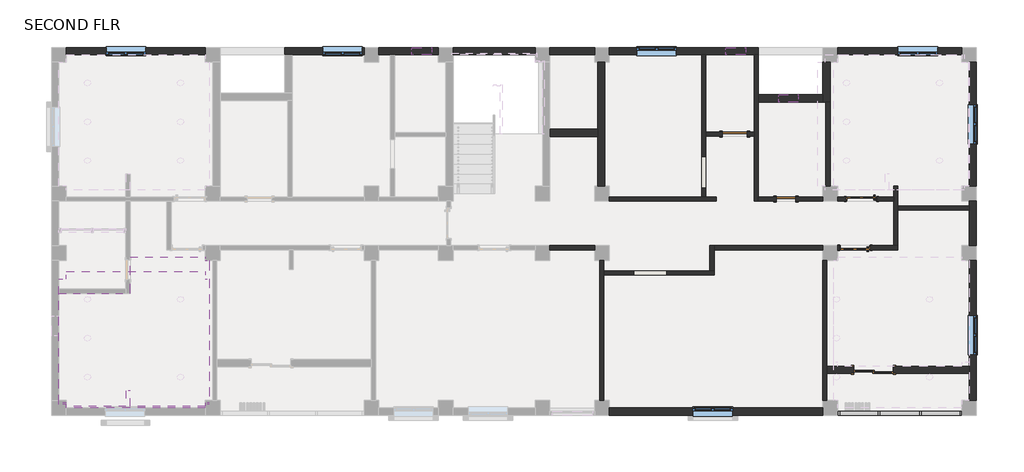
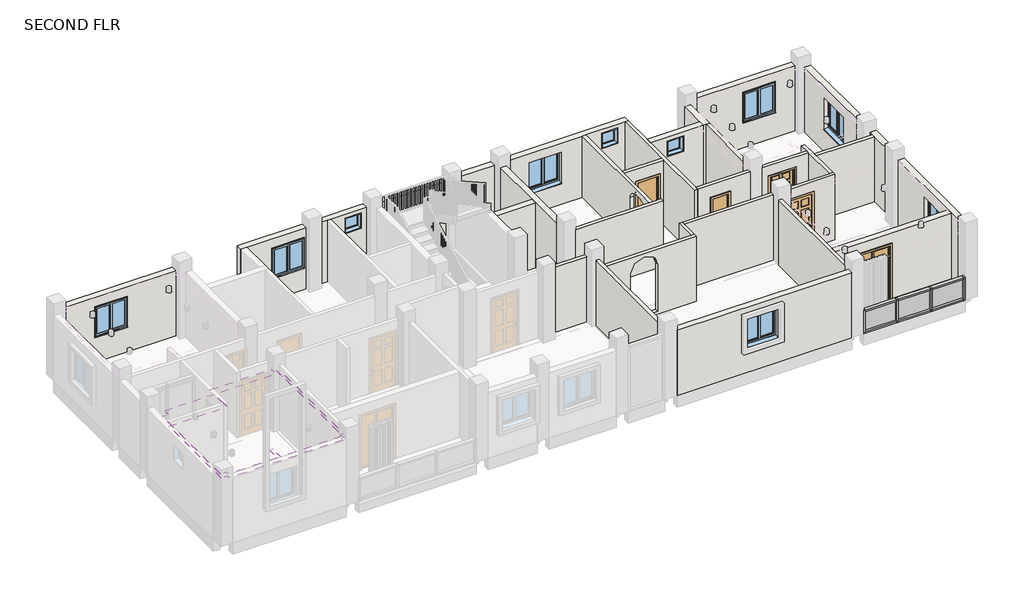
# One storey, part 2 of 5: 32 walls, 10 members, 10 windows, 5 doors, 3 plates, 2 coverings.
# Revit data of these elements (continued)
# Element 60 (IfcWindow, "w2.0001 : 4' X 4' WINDOW") (continued)
#   Materials on its faces: "Fenster - Kunststoff", "Fenster - Kunststoff weiss", "Glass", "Fenster - Holz"
# Element 61 (IfcWindow, "w2.0001 : 4' X 4' WINDOW")
#   Mark = "100"
#   Einbautiefe (von außen) = 0' - 5.51181"
#   Kippflügel = yes
#   Drehflügel im Grundriß darstellen = no
#   Drehflügel = yes
#   Rahmen = none
#   Glas = none
#   Flügel = none
#   Fensterbank innen = none
#   Fensterbank aussen = none
#   Phase Created = New Construction
#   Materials on its faces: "Fenster - Kunststoff", "Fenster - Kunststoff weiss", "Glass", "Fenster - Holz"
# Element 62 (IfcWindow, "w2.0001 : 4' X 4' WINDOW")
#   Mark = "106"
#   Einbautiefe (von außen) = 0' - 5.51181"
#   Kippflügel = yes
#   Drehflügel im Grundriß darstellen = no
#   Drehflügel = yes
#   Rahmen = none
#   Glas = none
#   Flügel = none
#   Fensterbank innen = none
#   Fensterbank aussen = none
#   Phase Created = New Construction
#   Materials on its faces: "Fenster - Kunststoff", "Fenster - Kunststoff weiss", "Glass", "Fenster - Holz"
# Materials
#   "WHITE CEILING 6\"": class "Generic", colour RGB 120 120 120, transparency 0, Cost = 0
#   "Glass": class "Glass", colour RGB 0 128 192, transparency 0.75, Description = "Soda Lime Glass", Cost = 0
#   "Wood - Birch - Solid Stained Light Low Gloss": class "Wood", colour RGB 210 159 95, transparency 0, Cost = 0
#   "Paint - Sienna": colour RGB 118 70 51, transparency 0, Cost = 0
#   "Cherry": class "Wood", colour RGB 226 177 128, transparency 0, Description = "Prunus Serotina", Cost = 0
#   "Aluminum": class "Metal", colour RGB 247 247 247, transparency 0, Description = "Aluminum 6061", Cost = 0
#   "Door - Panel": class "Wood", colour RGB 210 159 95, transparency 0, Cost = 0
#   "Door - Frame": colour RGB 118 70 51, transparency 0, Cost = 0
#   "SAND BEIGE PAINT": class "Generic", colour RGB 120 120 120, transparency 0, Cost = 0
#   "Sash": class "Wood", colour RGB 224 178 126, transparency 0, Cost = 0
#   "WINDOW FRAMING": class "Generic", colour RGB 120 120 120, transparency 0, Cost = 0
#   "Fenster - Kunststoff": colour RGB 249 249 249, transparency 0
#   "Fenster - Kunststoff weiss": colour RGB 249 249 249, transparency 0
#   "Fenster - Holz": colour RGB 216 135 75, transparency 0
